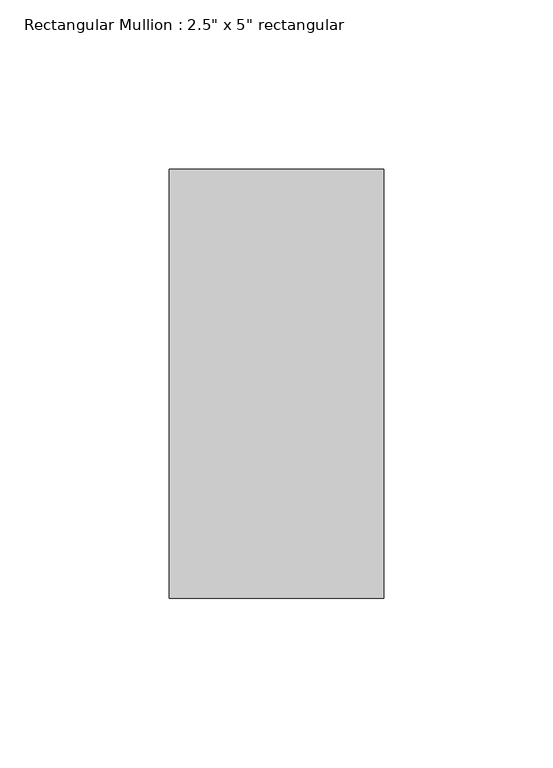
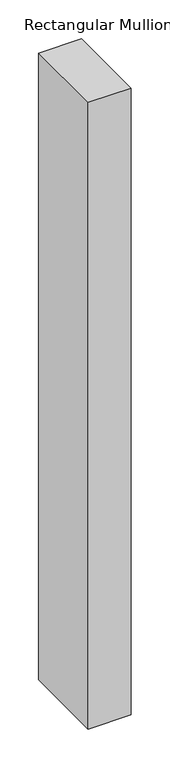
"""IFC4 building model written with IfcOpenShell, lengths in millimetres: member geometry."""

from ifc_helpers import new_model, si_unit, frame, origin, place, context, project, spatial, polyline, outline, extrude, source, transform, mapped, element, save


def member_09852e99(model_context):
    return source(origin(), model_context, "Body", "SweptSolid", [
        extrude(outline(polyline([(0.0, 63.5), (0.0, -63.5), (-63.5, -63.5), (-63.5, 63.5), (0.0, 63.5)])), frame((0.0, 0.0, -982.1333333), z_axis=(0.0, 0.0, 1.0), x_axis=(1.0, 0.0, 0.0)), (0.0, 0.0, 1.0), 982.1333333),
    ])


if __name__ == "__main__":
    model = new_model("IFC4")
    model_context = context("Model", 3, world=origin())
    ifc_project = project(units=[si_unit("LENGTHUNIT", "METRE", prefix="MILLI")], contexts=[model_context])
    site = spatial("IfcSite", under=ifc_project)
    building = spatial("IfcBuilding", under=site)
    placement = place(None, origin())
    member_shape = member_09852e99(model_context)
    element("IfcMember", 1, ObjectType="Rectangular Mullion : 2.5\" x 5\" rectangular", at=placement, inside=building, context=model_context, shape_type="MappedRepresentation", body=[
        mapped(member_shape, transform((0.0, 0.0, 0.0), x_axis=(1.0, 0.0, 0.0), y_axis=(0.0, 1.0, 0.0), z_axis=(0.0, 0.0, 1.0))),
    ])
    save(model, "model.ifc")

# Revit data of these elements
# Type "Rectangular Mullion : 2.5\" x 5\" rectangular"
#   built-in parameter 1007304 = 0.416667 (stored number, unit not read)
#   built-in parameter 1007301 = 0.104167 (stored number, unit not read)
#   built-in parameter 1007300 = 0.104167 (stored number, unit not read)
# Element 1 (IfcMember, "Rectangular Mullion : 2.5\" x 5\" rectangular")
#   Materials on its faces: "Aluminum"
# Materials
#   "Aluminum": class "Metal", colour RGB 247 247 247, transparency 0, Description = "Aluminum 6061", Cost = 0
